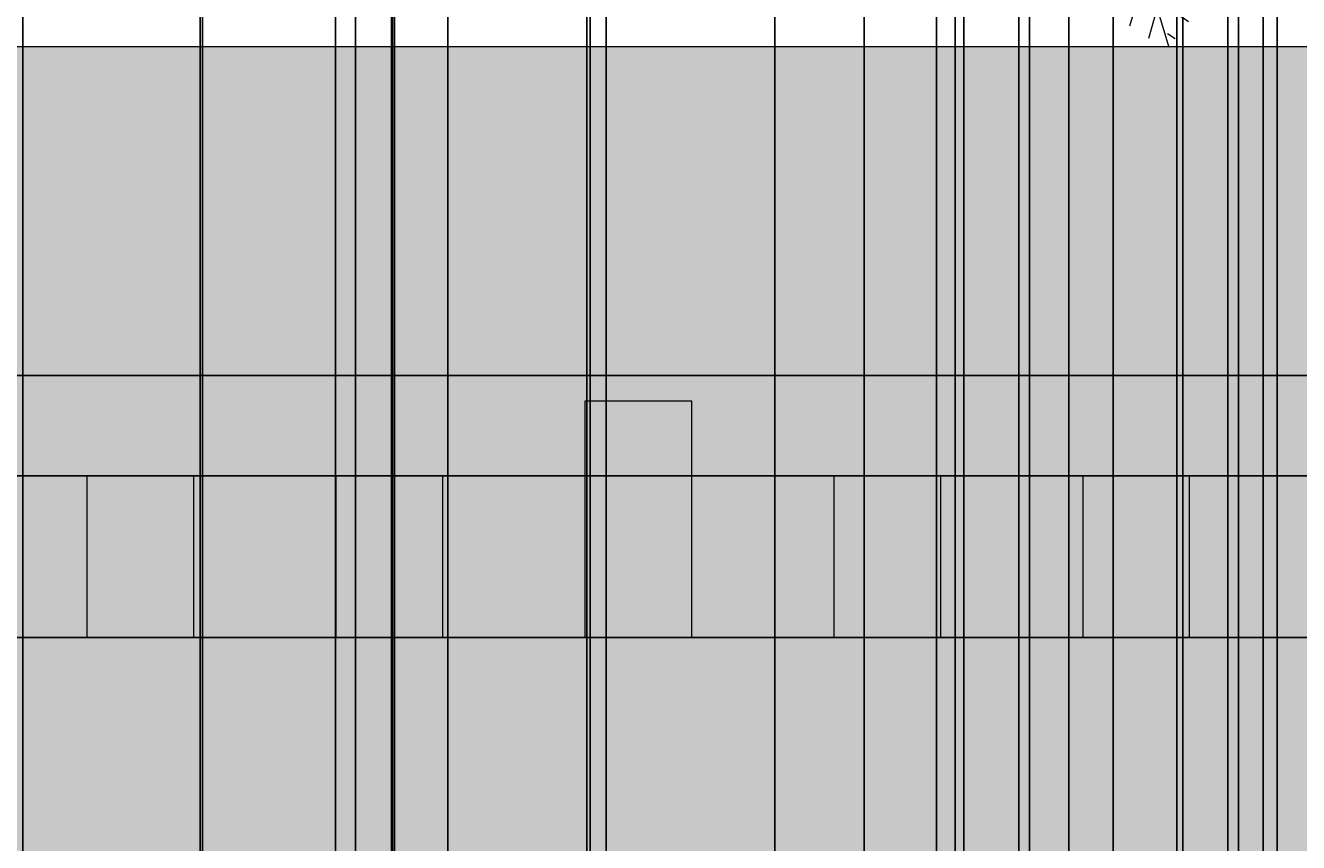
# Model space of a CAD drawing. Units: inches. Extents: x 818 to 1898, y 976 to 2364.
# Tile 80 of 96: x 1259 to 1439, y 2093 to 2209. Entities that reach past the tile are written whole.
import ezdxf

# ---------------------------------------------------------------- set-up
doc = ezdxf.new("R2010")
doc.units = ezdxf.units.IN
doc.header["$LTSCALE"] = 5
doc.header["$MEASUREMENT"] = 0
for name, color, linetype, lineweight in [('A-ANNO-DIMS', 2, 'Continuous', 18), ('L-PAVE', 8, 'Continuous', 18), ('L-PLNT-BEDS', 94, 'Continuous', 18)]:
    doc.layers.add(name, color=color, linetype=linetype, lineweight=lineweight)
for name, color, linetype, lineweight, true_color in [('L-PAVE-PATT', 9, 'Continuous', 9, 0xc7c8ca), ('L-PLNT', 116, 'Continuous', 13, 0x136734), ('L-PLNT-PATT', 114, 'Continuous', 9, 0x139b48)]:
    doc.layers.add(name, color=color, linetype=linetype, lineweight=lineweight, true_color=true_color)
doc.styles.get("Standard").update_dxf_attribs({"font": 'arial.ttf'})
doc.dimstyles.get("Standard").update_dxf_attribs({"dimtxt": 0.18, "dimasz": 0.18, "dimexe": 0.18, "dimexo": 0.0625, "dimgap": 0.09, "dimtad": 0, "dimtih": 1, "dimtoh": 1, "dimdec": 4, "dimzin": 0, "dimdsep": 46, "dimtxsty": 'Standard', "dimcen": 0.09, "dimadec": 0, "dimazin": 0, "dimtfac": 1, "dimtdec": 4, "dimtofl": 0, "dimtmove": 0, "dimatfit": 3, "dimfxl": 1, "dimtolj": 1, "dimtzin": 0, "dimarcsym": 0})

# ---------------------------------------------------------------- blocks, each defined once
blk = doc.blocks.new('PALM-BORDER')
for p, q in [((41.53, 39.05), (33.72, 81.45)), ((33.95, 78.95), (31.8, 80.68)), ((34.76, 77.57), (36.65, 80.68)), ((35.03, 74.11), (28.83, 78.26)), ((35.84, 71.35), (39.61, 75.84)), ((37.18, 65.82), (45, 74.8)), ((36.11, 68.59), (25.33, 73.77)), ((37.72, 59.6), (49.31, 73.77)), ((37.72, 59.95), (23.17, 69.28)), ((39.34, 51.31), (47.96, 67.2)), ((38.8, 53.39), (21.02, 65.48)), ((61.61, 45.75), (77.23, 65.83)), ((61.71, 45.79), (64.67, 65.82)), ((74.37, 66.17), (75.18, 63.4)), ((57.93, 44.41), (61.97, 63.06)), ((67.63, 63.4), (69.25, 55.81)), ((70.33, 64.44), (72.75, 60.3)), ((53.62, 43.37), (58.74, 62.37)), ((65.21, 62.02), (65.75, 51.31)), ((74.1, 61.33), (79.49, 62.02)), ((5.39, 54.77), (4.85, 60.64)), ((9.16, 60.3), (9.97, 50.62)), ((15.09, 59.95), (23.44, 41.99)), ((18.1, 42.4), (2.48, 58.02)), ((12.93, 58.57), (15.63, 44.75)), ((30.72, 40.61), (18.59, 57.88)), ((40.69, 44.06), (48.23, 58.91)), ((49.04, 41.64), (54.7, 58.57)), ((71.68, 58.22), (77.87, 57.53)), ((23.44, 56.84), (39.34, 49.24)), ((44.46, 40.26), (49.85, 57.19)), ((6.2, 53.73), (0, 52.7)), ((68.44, 53.73), (77.33, 52.35)), ((66.29, 51.31), (77.87, 47.17)), ((11.32, 49.24), (0.54, 47.17)), ((26.14, 49.24), (40.69, 42.68)), ((63.59, 48.21), (77.33, 43.71)), ((41.53, 39.05), (61.61, 45.75)), ((16.71, 43.71), (2.69, 43.02)), ((54.97, 43.37), (67.63, 36.46)), ((59.55, 44.75), (76.26, 40.26)), ((20.48, 41.64), (5.93, 34.73)), ((41.53, 39.05), (18.1, 42.4)), ((49.85, 41.64), (64.4, 34.73)), ((25.6, 41.3), (13.2, 33.01)), ((29.64, 40.61), (19.13, 31.97)), ((36.65, 39.91), (25.6, 33.01)), ((46.35, 40.26), (60.9, 32.66)), ((41.53, 39.05), (24.79, 24.55)), ((41.53, 39.05), (54.92, 22.32)), ((37.99, 36.46), (38.8, 28.17)), ((43.38, 36.81), (40.42, 24.02)), ((42.84, 37.15), (59.55, 31.97)), ((36.65, 34.73), (26.68, 31.62)), ((45.27, 34.39), (43.11, 19.88)), ((34.49, 32.66), (36.92, 21.61)), ((47.15, 32.32), (65.48, 28.17)), ((30.18, 29.55), (19.13, 29.55)), ((31.53, 30.59), (35.03, 14.7)), ((48.23, 30.59), (44.19, 12.28)), ((28.56, 27.82), (9.7, 25.06)), ((28.83, 27.82), (32.07, 9.17)), ((50.66, 27.82), (68.98, 25.06)), ((26.14, 25.41), (28.29, 6.06)), ((52, 26.44), (46.35, 9.17)), ((24.79, 24.55), (13.63, 5.58)), ((53.62, 24.37), (68.44, 21.95)), ((23.44, 22.99), (9.97, 22.64)), ((54.97, 22.3), (47.69, 5.02)), ((54.92, 22.32), (61.61, 0)), ((55.24, 22.3), (71.68, 17.46)), ((21.56, 19.53), (11.59, 19.88)), ((22.9, 21.26), (24.52, 5.37)), ((55.78, 20.22), (70.33, 14.35)), ((20.48, 17.46), (9.7, 15.73)), ((56.59, 16.42), (53.35, 5.72)), ((19.94, 16.08), (20.75, 6.41)), ((57.39, 14.7), (70.6, 8.83)), ((18.59, 13.66), (9.97, 12.62)), ((17.24, 11.59), (17.78, 6.06)), ((58.47, 10.9), (56.05, 2.95)), ((15.9, 9.52), (11.05, 7.44)), ((58.47, 10.55), (67.09, 5.72)), ((59.82, 6.75), (64.4, 3.64)), ((59.82, 5.02), (58.74, 1.22)), ((61.44, 1.92), (62.51, 1.22))]:
    blk.add_line(p, q)
blk = doc.blocks.new('*D61')
at = {"layer": 'A-ANNO-DIMS', "color": 0, "lineweight": -2, "ltscale": 5, "transparency": 16777216}
for p, q in [((1071.73, 1203.03), (1071.73, 2363.87)), ((1071.91, 2363.69), (1250.94, 2363.69)), ((1430.55, 2363.69), (1251.51, 2363.69)), ((1430.73, 1203.03), (1430.73, 2363.87))]:
    blk.add_line(p, q, dxfattribs=at)
at = {"layer": 'A-ANNO-DIMS', "color": 0, "ltscale": 5, "transparency": 16777216}
for points in [[(1071.91, 2363.72), (1071.91, 2363.66), (1071.73, 2363.69)], [(1430.55, 2363.72), (1430.55, 2363.66), (1430.73, 2363.69)]]:
    blk.add_solid(points, dxfattribs=at)
at = {"layer": 'Defpoints', "color": 0, "ltscale": 5, "transparency": 16777216}
for p in [(1430.73, 2363.69), (1071.73, 1202.96), (1430.73, 1202.96)]:
    blk.add_point(p, dxfattribs=at)
at = {"layer": 'A-ANNO-DIMS', "color": 0, "ltscale": 5, "transparency": 16777216, "insert": (1251.23, 2363.69), "char_height": 0.18, "attachment_point": 5}
blk.add_mtext('\\A1;359', dxfattribs=at)
blk = doc.blocks.new('*D64')
at = {"layer": 'A-ANNO-DIMS', "color": 0, "lineweight": -2, "ltscale": 5, "transparency": 16777216}
for p, q in [((1197.73, 1501.14), (1197.73, 2363.87)), ((1197.91, 2363.69), (1313.93, 2363.69)), ((1430.55, 2363.69), (1314.52, 2363.69)), ((1430.73, 1501.14), (1430.73, 2363.87))]:
    blk.add_line(p, q, dxfattribs=at)
at = {"layer": 'A-ANNO-DIMS', "color": 0, "ltscale": 5, "transparency": 16777216}
for points in [[(1197.91, 2363.72), (1197.91, 2363.66), (1197.73, 2363.69)], [(1430.55, 2363.72), (1430.55, 2363.66), (1430.73, 2363.69)]]:
    blk.add_solid(points, dxfattribs=at)
at = {"layer": 'Defpoints', "color": 0, "ltscale": 5, "transparency": 16777216}
for p in [(1430.73, 2363.69), (1197.73, 1501.08), (1430.73, 1501.08)]:
    blk.add_point(p, dxfattribs=at)
at = {"layer": 'A-ANNO-DIMS', "color": 0, "ltscale": 5, "transparency": 16777216, "insert": (1314.23, 2363.69), "char_height": 0.18, "attachment_point": 5}
blk.add_mtext('\\A1;233', dxfattribs=at)
blk = doc.blocks.new('*D86')
at = {"layer": 'A-ANNO-DIMS', "color": 0, "lineweight": -2, "ltscale": 5, "transparency": 16777216}
for p, q in [((1258.73, 2053.14), (1258.73, 2363.87)), ((1258.91, 2363.69), (1486.43, 2363.69)), ((1714.55, 2363.69), (1487.02, 2363.69)), ((1714.73, 2053.14), (1714.73, 2363.87))]:
    blk.add_line(p, q, dxfattribs=at)
at = {"layer": 'A-ANNO-DIMS', "color": 0, "ltscale": 5, "transparency": 16777216}
for points in [[(1258.91, 2363.72), (1258.91, 2363.66), (1258.73, 2363.69)], [(1714.55, 2363.72), (1714.55, 2363.66), (1714.73, 2363.69)]]:
    blk.add_solid(points, dxfattribs=at)
at = {"layer": 'Defpoints', "color": 0, "ltscale": 5, "transparency": 16777216}
for p in [(1714.73, 2363.69), (1258.73, 2053.08), (1714.73, 2053.08)]:
    blk.add_point(p, dxfattribs=at)
at = {"layer": 'A-ANNO-DIMS', "color": 0, "ltscale": 5, "transparency": 16777216, "insert": (1486.73, 2363.69), "char_height": 0.18, "attachment_point": 5}
blk.add_mtext('\\A1;456', dxfattribs=at)
blk = doc.blocks.new('*D96')
at = {"layer": 'A-ANNO-DIMS', "color": 0, "lineweight": -2, "ltscale": 5, "transparency": 16777216}
for p, q in [((1229.65, 1071.12), (1229.65, 2363.87)), ((1229.83, 2363.69), (1256.52, 2363.69)), ((1283.99, 2363.69), (1257.3, 2363.69)), ((1284.17, 1071.12), (1284.17, 2363.87))]:
    blk.add_line(p, q, dxfattribs=at)
at = {"layer": 'A-ANNO-DIMS', "color": 0, "ltscale": 5, "transparency": 16777216}
for points in [[(1229.83, 2363.72), (1229.83, 2363.66), (1229.65, 2363.69)], [(1283.99, 2363.72), (1283.99, 2363.66), (1284.17, 2363.69)]]:
    blk.add_solid(points, dxfattribs=at)
at = {"layer": 'Defpoints', "color": 0, "ltscale": 5, "transparency": 16777216}
for p in [(1284.17, 2363.69), (1229.65, 1071.06), (1284.17, 1071.06)]:
    blk.add_point(p, dxfattribs=at)
at = {"layer": 'A-ANNO-DIMS', "color": 0, "ltscale": 5, "transparency": 16777216, "insert": (1256.91, 2363.69), "char_height": 0.18, "attachment_point": 5}
blk.add_mtext('\\A1;54.52', dxfattribs=at)
blk = doc.blocks.new('*D97')
at = {"layer": 'A-ANNO-DIMS', "color": 0, "lineweight": -2, "ltscale": 5, "transparency": 16777216}
for p, q in [((1284.17, 1071.12), (1284.17, 2363.87)), ((1284.35, 2363.69), (1310.96, 2363.69)), ((1338.36, 2363.69), (1311.75, 2363.69)), ((1338.54, 1071.12), (1338.54, 2363.87))]:
    blk.add_line(p, q, dxfattribs=at)
at = {"layer": 'A-ANNO-DIMS', "color": 0, "ltscale": 5, "transparency": 16777216}
for points in [[(1284.35, 2363.72), (1284.35, 2363.66), (1284.17, 2363.69)], [(1338.36, 2363.72), (1338.36, 2363.66), (1338.54, 2363.69)]]:
    blk.add_solid(points, dxfattribs=at)
at = {"layer": 'Defpoints', "color": 0, "ltscale": 5, "transparency": 16777216}
for p in [(1338.54, 2363.69), (1284.17, 1071.06), (1338.54, 1071.06)]:
    blk.add_point(p, dxfattribs=at)
at = {"layer": 'A-ANNO-DIMS', "color": 0, "ltscale": 5, "transparency": 16777216, "insert": (1311.36, 2363.69), "char_height": 0.18, "attachment_point": 5}
blk.add_mtext('\\A1;54.37', dxfattribs=at)
blk = doc.blocks.new('*D98')
at = {"layer": 'A-ANNO-DIMS', "color": 0, "lineweight": -2, "ltscale": 5, "transparency": 16777216}
for p, q in [((1338.54, 1071.12), (1338.54, 2363.87)), ((1338.72, 2363.69), (1364.81, 2363.69)), ((1391.7, 2363.69), (1365.6, 2363.69)), ((1391.88, 1071.12), (1391.88, 2363.87))]:
    blk.add_line(p, q, dxfattribs=at)
at = {"layer": 'A-ANNO-DIMS', "color": 0, "ltscale": 5, "transparency": 16777216}
for points in [[(1338.72, 2363.72), (1338.72, 2363.66), (1338.54, 2363.69)], [(1391.7, 2363.72), (1391.7, 2363.66), (1391.88, 2363.69)]]:
    blk.add_solid(points, dxfattribs=at)
at = {"layer": 'Defpoints', "color": 0, "ltscale": 5, "transparency": 16777216}
for p in [(1391.88, 2363.69), (1338.54, 1071.06), (1391.88, 1071.06)]:
    blk.add_point(p, dxfattribs=at)
at = {"layer": 'A-ANNO-DIMS', "color": 0, "ltscale": 5, "transparency": 16777216, "insert": (1365.21, 2363.69), "char_height": 0.18, "attachment_point": 5}
blk.add_mtext('\\A1;53.33', dxfattribs=at)
blk = doc.blocks.new('*D99')
at = {"layer": 'A-ANNO-DIMS', "color": 0, "lineweight": -2, "ltscale": 5, "transparency": 16777216}
for p, q in [((1391.88, 1071.12), (1391.88, 2363.87)), ((1392.06, 2363.69), (1420.45, 2363.69)), ((1449.64, 2363.69), (1421.24, 2363.69)), ((1449.82, 1071.12), (1449.82, 2363.87))]:
    blk.add_line(p, q, dxfattribs=at)
at = {"layer": 'A-ANNO-DIMS', "color": 0, "ltscale": 5, "transparency": 16777216}
for points in [[(1392.06, 2363.72), (1392.06, 2363.66), (1391.88, 2363.69)], [(1449.64, 2363.72), (1449.64, 2363.66), (1449.82, 2363.69)]]:
    blk.add_solid(points, dxfattribs=at)
at = {"layer": 'Defpoints', "color": 0, "ltscale": 5, "transparency": 16777216}
for p in [(1449.82, 2363.69), (1391.88, 1071.06), (1449.82, 1071.06)]:
    blk.add_point(p, dxfattribs=at)
at = {"layer": 'A-ANNO-DIMS', "color": 0, "ltscale": 5, "transparency": 16777216, "insert": (1420.85, 2363.69), "char_height": 0.18, "attachment_point": 5}
blk.add_mtext('\\A1;57.94', dxfattribs=at)
blk = doc.blocks.new('*D147')
at = {"layer": 'A-ANNO-DIMS', "color": 0, "lineweight": -2, "ltscale": 5, "transparency": 16777216}
for p, q in [((1212.58, 2145.25), (1897.92, 2145.25)), ((1897.74, 2145.07), (1897.74, 2133.99)), ((1897.74, 2122.56), (1897.74, 2133.63)), ((1212.58, 2122.38), (1897.92, 2122.38))]:
    blk.add_line(p, q, dxfattribs=at)
at = {"layer": 'A-ANNO-DIMS', "color": 0, "ltscale": 5, "transparency": 16777216}
for points in [[(1897.71, 2145.07), (1897.77, 2145.07), (1897.74, 2145.25)], [(1897.71, 2122.56), (1897.77, 2122.56), (1897.74, 2122.38)]]:
    blk.add_solid(points, dxfattribs=at)
at = {"layer": 'Defpoints', "color": 0, "ltscale": 5, "transparency": 16777216}
for p in [(1212.52, 2145.25), (1897.74, 2145.25), (1212.52, 2122.38)]:
    blk.add_point(p, dxfattribs=at)
at = {"layer": 'A-ANNO-DIMS', "color": 0, "ltscale": 5, "transparency": 16777216, "insert": (1897.74, 2133.81), "char_height": 0.18, "attachment_point": 5}
blk.add_mtext('\\A1;22.87', dxfattribs=at)
blk = doc.blocks.new('*D148')
at = {"layer": 'A-ANNO-DIMS', "color": 0, "lineweight": -2, "ltscale": 5, "transparency": 16777216}
for p, q in [((1232.67, 2159.43), (1897.92, 2159.43)), ((1897.74, 2159.25), (1897.74, 2141.09)), ((1897.74, 2122.56), (1897.74, 2140.72)), ((1232.67, 2122.38), (1897.92, 2122.38))]:
    blk.add_line(p, q, dxfattribs=at)
at = {"layer": 'A-ANNO-DIMS', "color": 0, "ltscale": 5, "transparency": 16777216}
for points in [[(1897.71, 2159.25), (1897.77, 2159.25), (1897.74, 2159.43)], [(1897.71, 2122.56), (1897.77, 2122.56), (1897.74, 2122.38)]]:
    blk.add_solid(points, dxfattribs=at)
at = {"layer": 'Defpoints', "color": 0, "ltscale": 5, "transparency": 16777216}
for p in [(1232.61, 2159.43), (1897.74, 2159.43), (1232.61, 2122.38)]:
    blk.add_point(p, dxfattribs=at)
at = {"layer": 'A-ANNO-DIMS', "color": 0, "ltscale": 5, "transparency": 16777216, "insert": (1897.74, 2140.9), "char_height": 0.18, "attachment_point": 5}
blk.add_mtext('\\A1;37.05', dxfattribs=at)
blk = doc.blocks.new('*D161')
at = {"layer": 'A-ANNO-DIMS', "color": 0, "lineweight": -2, "ltscale": 5, "transparency": 16777216}
for p, q in [((1429.23, 1876.14), (1429.23, 2363.87)), ((1429.41, 2363.69), (1509.59, 2363.69)), ((1590.55, 2363.69), (1510.36, 2363.69)), ((1590.73, 1876.14), (1590.73, 2363.87))]:
    blk.add_line(p, q, dxfattribs=at)
at = {"layer": 'A-ANNO-DIMS', "color": 0, "ltscale": 5, "transparency": 16777216}
for points in [[(1429.41, 2363.72), (1429.41, 2363.66), (1429.23, 2363.69)], [(1590.55, 2363.72), (1590.55, 2363.66), (1590.73, 2363.69)]]:
    blk.add_solid(points, dxfattribs=at)
at = {"layer": 'Defpoints', "color": 0, "ltscale": 5, "transparency": 16777216}
for p in [(1590.73, 2363.69), (1429.23, 1876.08), (1590.73, 1876.08)]:
    blk.add_point(p, dxfattribs=at)
at = {"layer": 'A-ANNO-DIMS', "color": 0, "ltscale": 5, "transparency": 16777216, "insert": (1509.98, 2363.69), "char_height": 0.18, "attachment_point": 5}
blk.add_mtext('\\A1;161.5', dxfattribs=at)
blk = doc.blocks.new('*D165')
at = {"layer": 'A-ANNO-DIMS', "color": 0, "lineweight": -2, "ltscale": 5, "transparency": 16777216}
for p, q in [((1283.82, 1510.14), (1283.82, 2363.87)), ((1284, 2363.69), (1324.09, 2363.69)), ((1364.97, 2363.69), (1324.88, 2363.69)), ((1365.15, 1510.14), (1365.15, 2363.87))]:
    blk.add_line(p, q, dxfattribs=at)
at = {"layer": 'A-ANNO-DIMS', "color": 0, "ltscale": 5, "transparency": 16777216}
for points in [[(1284, 2363.72), (1284, 2363.66), (1283.82, 2363.69)], [(1364.97, 2363.72), (1364.97, 2363.66), (1365.15, 2363.69)]]:
    blk.add_solid(points, dxfattribs=at)
at = {"layer": 'Defpoints', "color": 0, "ltscale": 5, "transparency": 16777216}
for p in [(1365.15, 2363.69), (1283.82, 1510.08), (1365.15, 1510.08)]:
    blk.add_point(p, dxfattribs=at)
at = {"layer": 'A-ANNO-DIMS', "color": 0, "ltscale": 5, "transparency": 16777216, "insert": (1324.48, 2363.69), "char_height": 0.18, "attachment_point": 5}
blk.add_mtext('\\A1;81.33', dxfattribs=at)
blk = doc.blocks.new('*D166')
at = {"layer": 'A-ANNO-DIMS', "color": 0, "lineweight": -2, "ltscale": 5, "transparency": 16777216}
for p, q in [((1401.15, 1510.14), (1401.15, 2363.87)), ((1401.33, 2363.69), (1415.54, 2363.69)), ((1430.55, 2363.69), (1416.33, 2363.69)), ((1430.73, 1510.14), (1430.73, 2363.87))]:
    blk.add_line(p, q, dxfattribs=at)
at = {"layer": 'A-ANNO-DIMS', "color": 0, "ltscale": 5, "transparency": 16777216}
for points in [[(1401.33, 2363.72), (1401.33, 2363.66), (1401.15, 2363.69)], [(1430.55, 2363.72), (1430.55, 2363.66), (1430.73, 2363.69)]]:
    blk.add_solid(points, dxfattribs=at)
at = {"layer": 'Defpoints', "color": 0, "ltscale": 5, "transparency": 16777216}
for p in [(1430.73, 2363.69), (1401.15, 1510.08), (1430.73, 1510.08)]:
    blk.add_point(p, dxfattribs=at)
at = {"layer": 'A-ANNO-DIMS', "color": 0, "ltscale": 5, "transparency": 16777216, "insert": (1415.94, 2363.69), "char_height": 0.18, "attachment_point": 5}
blk.add_mtext('\\A1;29.58', dxfattribs=at)
blk = doc.blocks.new('*D191')
at = {"layer": 'A-ANNO-DIMS', "color": 0, "lineweight": -2, "ltscale": 5, "transparency": 16777216}
for p, q in [((1434.23, 1409.11), (1434.23, 2363.87)), ((1434.41, 2363.69), (1435.08, 2363.69)), ((1436.05, 2363.69), (1435.37, 2363.69)), ((1436.23, 1409.11), (1436.23, 2363.87))]:
    blk.add_line(p, q, dxfattribs=at)
at = {"layer": 'A-ANNO-DIMS', "color": 0, "ltscale": 5, "transparency": 16777216}
for points in [[(1434.41, 2363.72), (1434.41, 2363.66), (1434.23, 2363.69)], [(1436.05, 2363.72), (1436.05, 2363.66), (1436.23, 2363.69)]]:
    blk.add_solid(points, dxfattribs=at)
at = {"layer": 'Defpoints', "color": 0, "ltscale": 5, "transparency": 16777216}
for p in [(1436.23, 2363.69), (1434.23, 1409.05), (1436.23, 1409.05)]:
    blk.add_point(p, dxfattribs=at)
at = {"layer": 'A-ANNO-DIMS', "color": 0, "ltscale": 5, "transparency": 16777216, "insert": (1435.23, 2363.69), "char_height": 0.18, "attachment_point": 5}
blk.add_mtext('\\A1;2', dxfattribs=at)
blk = doc.blocks.new('*D235')
at = {"layer": 'A-ANNO-DIMS', "color": 0, "lineweight": -2, "ltscale": 5, "transparency": 16777216}
for p, q in [((1310.91, 2026.27), (1310.91, 2363.87)), ((1311.09, 2363.69), (1324.48, 2363.69)), ((1338.81, 2363.69), (1325.41, 2363.69)), ((1338.99, 2026.27), (1338.99, 2363.87))]:
    blk.add_line(p, q, dxfattribs=at)
at = {"layer": 'A-ANNO-DIMS', "color": 0, "ltscale": 5, "transparency": 16777216}
for points in [[(1311.09, 2363.72), (1311.09, 2363.66), (1310.91, 2363.69)], [(1338.81, 2363.72), (1338.81, 2363.66), (1338.99, 2363.69)]]:
    blk.add_solid(points, dxfattribs=at)
at = {"layer": 'Defpoints', "color": 0, "ltscale": 5, "transparency": 16777216}
for p in [(1338.99, 2363.69), (1310.91, 2026.21), (1338.99, 2026.21)]:
    blk.add_point(p, dxfattribs=at)
at = {"layer": 'A-ANNO-DIMS', "color": 0, "ltscale": 5, "transparency": 16777216, "insert": (1324.95, 2363.69), "char_height": 0.18, "attachment_point": 5}
blk.add_mtext('\\A1;28.084', dxfattribs=at)
blk = doc.blocks.new('*D255')
at = {"layer": 'A-ANNO-DIMS', "color": 0, "lineweight": -2, "ltscale": 5, "transparency": 16777216}
for p, q in [((1388.03, 2053.14), (1388.03, 2363.87)), ((1388.21, 2363.69), (1388.94, 2363.69)), ((1390.46, 2363.69), (1389.73, 2363.69)), ((1390.64, 2053.14), (1390.64, 2363.87))]:
    blk.add_line(p, q, dxfattribs=at)
at = {"layer": 'A-ANNO-DIMS', "color": 0, "ltscale": 5, "transparency": 16777216}
for points in [[(1388.21, 2363.72), (1388.21, 2363.66), (1388.03, 2363.69)], [(1390.46, 2363.72), (1390.46, 2363.66), (1390.64, 2363.69)]]:
    blk.add_solid(points, dxfattribs=at)
at = {"layer": 'Defpoints', "color": 0, "ltscale": 5, "transparency": 16777216}
for p in [(1390.64, 2363.69), (1388.03, 2053.08), (1390.64, 2053.08)]:
    blk.add_point(p, dxfattribs=at)
at = {"layer": 'A-ANNO-DIMS', "color": 0, "ltscale": 5, "transparency": 16777216, "insert": (1389.33, 2363.69), "char_height": 0.18, "attachment_point": 5}
blk.add_mtext('\\A1;2.604', dxfattribs=at)
blk = doc.blocks.new('*D256')
at = {"layer": 'A-ANNO-DIMS', "color": 0, "lineweight": -2, "ltscale": 5, "transparency": 16777216}
for p, q in [((1399.64, 2053.14), (1399.64, 2363.87)), ((1399.82, 2363.69), (1405.87, 2363.69)), ((1412.84, 2363.69), (1406.78, 2363.69)), ((1413.02, 2077.25), (1413.02, 2363.87))]:
    blk.add_line(p, q, dxfattribs=at)
at = {"layer": 'A-ANNO-DIMS', "color": 0, "ltscale": 5, "transparency": 16777216}
for points in [[(1399.82, 2363.72), (1399.82, 2363.66), (1399.64, 2363.69)], [(1412.84, 2363.72), (1412.84, 2363.66), (1413.02, 2363.69)]]:
    blk.add_solid(points, dxfattribs=at)
at = {"layer": 'Defpoints', "color": 0, "ltscale": 5, "transparency": 16777216}
for p in [(1413.02, 2363.69), (1413.02, 2077.19), (1399.64, 2053.08)]:
    blk.add_point(p, dxfattribs=at)
at = {"layer": 'A-ANNO-DIMS', "color": 0, "ltscale": 5, "transparency": 16777216, "insert": (1406.33, 2363.69), "char_height": 0.18, "attachment_point": 5}
blk.add_mtext('\\A1;13.384', dxfattribs=at)
blk = doc.blocks.new('*D258')
at = {"layer": 'A-ANNO-DIMS', "color": 0, "lineweight": -2, "ltscale": 5, "transparency": 16777216}
for p, q in [((1422.02, 2053.14), (1422.02, 2363.87)), ((1422.2, 2363.69), (1453.26, 2363.69)), ((1484.94, 2363.69), (1453.88, 2363.69)), ((1485.12, 2053.14), (1485.12, 2363.87))]:
    blk.add_line(p, q, dxfattribs=at)
at = {"layer": 'A-ANNO-DIMS', "color": 0, "ltscale": 5, "transparency": 16777216}
for points in [[(1422.2, 2363.72), (1422.2, 2363.66), (1422.02, 2363.69)], [(1484.94, 2363.72), (1484.94, 2363.66), (1485.12, 2363.69)]]:
    blk.add_solid(points, dxfattribs=at)
at = {"layer": 'Defpoints', "color": 0, "ltscale": 5, "transparency": 16777216}
for p in [(1485.12, 2363.69), (1422.02, 2053.08), (1485.12, 2053.08)]:
    blk.add_point(p, dxfattribs=at)
at = {"layer": 'A-ANNO-DIMS', "color": 0, "ltscale": 5, "transparency": 16777216, "insert": (1453.57, 2363.69), "char_height": 0.18, "attachment_point": 5}
blk.add_mtext('\\A1;63.1', dxfattribs=at)
blk = doc.blocks.new('*D269')
at = {"layer": 'A-ANNO-DIMS', "color": 0, "lineweight": -2, "ltscale": 5, "transparency": 16777216}
for p, q in [((1246.94, 1534.14), (1246.94, 2363.87)), ((1247.12, 2363.69), (1293.71, 2363.69)), ((1341.08, 2363.69), (1294.49, 2363.69)), ((1341.26, 1534.14), (1341.26, 2363.87))]:
    blk.add_line(p, q, dxfattribs=at)
at = {"layer": 'A-ANNO-DIMS', "color": 0, "ltscale": 5, "transparency": 16777216}
for points in [[(1247.12, 2363.72), (1247.12, 2363.66), (1246.94, 2363.69)], [(1341.08, 2363.72), (1341.08, 2363.66), (1341.26, 2363.69)]]:
    blk.add_solid(points, dxfattribs=at)
at = {"layer": 'Defpoints', "color": 0, "ltscale": 5, "transparency": 16777216}
for p in [(1341.26, 2363.69), (1246.94, 1534.08), (1341.26, 1534.08)]:
    blk.add_point(p, dxfattribs=at)
at = {"layer": 'A-ANNO-DIMS', "color": 0, "ltscale": 5, "transparency": 16777216, "insert": (1294.1, 2363.69), "char_height": 0.18, "attachment_point": 5}
blk.add_mtext('\\A1;94.32', dxfattribs=at)
blk = doc.blocks.new('*D273')
at = {"layer": 'A-ANNO-DIMS', "color": 0, "lineweight": -2, "ltscale": 5, "transparency": 16777216}
for p, q in [((1406.73, 1587.48), (1406.73, 2363.87)), ((1406.91, 2363.69), (1418.51, 2363.69)), ((1430.55, 2363.69), (1418.95, 2363.69)), ((1430.73, 1587.48), (1430.73, 2363.87))]:
    blk.add_line(p, q, dxfattribs=at)
at = {"layer": 'A-ANNO-DIMS', "color": 0, "ltscale": 5, "transparency": 16777216}
for points in [[(1406.91, 2363.72), (1406.91, 2363.66), (1406.73, 2363.69)], [(1430.55, 2363.72), (1430.55, 2363.66), (1430.73, 2363.69)]]:
    blk.add_solid(points, dxfattribs=at)
at = {"layer": 'Defpoints', "color": 0, "ltscale": 5, "transparency": 16777216}
for p in [(1430.73, 2363.69), (1406.73, 1587.42), (1430.73, 1587.42)]:
    blk.add_point(p, dxfattribs=at)
at = {"layer": 'A-ANNO-DIMS', "color": 0, "ltscale": 5, "transparency": 16777216, "insert": (1418.73, 2363.69), "char_height": 0.18, "attachment_point": 5}
blk.add_mtext('\\A1;24', dxfattribs=at)
blk = doc.blocks.new('*D274')
at = {"layer": 'A-ANNO-DIMS', "color": 0, "lineweight": -2, "ltscale": 5, "transparency": 16777216}
for p, q in [((1311.03, 1897.93), (1311.03, 2363.87)), ((1311.21, 2363.69), (1344.01, 2363.69)), ((1377.6, 2363.69), (1344.8, 2363.69)), ((1377.78, 1897.93), (1377.78, 2363.87))]:
    blk.add_line(p, q, dxfattribs=at)
at = {"layer": 'A-ANNO-DIMS', "color": 0, "ltscale": 5, "transparency": 16777216}
for points in [[(1311.21, 2363.72), (1311.21, 2363.66), (1311.03, 2363.69)], [(1377.6, 2363.72), (1377.6, 2363.66), (1377.78, 2363.69)]]:
    blk.add_solid(points, dxfattribs=at)
at = {"layer": 'Defpoints', "color": 0, "ltscale": 5, "transparency": 16777216}
for p in [(1377.78, 2363.69), (1311.03, 1897.87), (1377.78, 1897.87)]:
    blk.add_point(p, dxfattribs=at)
at = {"layer": 'A-ANNO-DIMS', "color": 0, "ltscale": 5, "transparency": 16777216, "insert": (1344.4, 2363.69), "char_height": 0.18, "attachment_point": 5}
blk.add_mtext('\\A1;66.75', dxfattribs=at)
blk = doc.blocks.new('*D281')
at = {"layer": 'A-ANNO-DIMS', "color": 0, "lineweight": -2, "ltscale": 5, "transparency": 16777216}
for p, q in [((1250.3, 1913.7), (1250.3, 2363.87)), ((1250.48, 2363.69), (1420.12, 2363.69)), ((1590.55, 2363.69), (1420.91, 2363.69)), ((1590.73, 2011.14), (1590.73, 2363.87))]:
    blk.add_line(p, q, dxfattribs=at)
at = {"layer": 'A-ANNO-DIMS', "color": 0, "ltscale": 5, "transparency": 16777216}
for points in [[(1250.48, 2363.72), (1250.48, 2363.66), (1250.3, 2363.69)], [(1590.55, 2363.72), (1590.55, 2363.66), (1590.73, 2363.69)]]:
    blk.add_solid(points, dxfattribs=at)
at = {"layer": 'Defpoints', "color": 0, "ltscale": 5, "transparency": 16777216}
for p in [(1590.73, 2363.69), (1590.73, 2011.08), (1250.3, 1913.64)]:
    blk.add_point(p, dxfattribs=at)
at = {"layer": 'A-ANNO-DIMS', "color": 0, "ltscale": 5, "transparency": 16777216, "insert": (1420.51, 2363.69), "char_height": 0.18, "attachment_point": 5}
blk.add_mtext('\\A1;340.4', dxfattribs=at)
blk = doc.blocks.new('*D286')
at = {"layer": 'A-ANNO-DIMS', "color": 0, "lineweight": -2, "ltscale": 5, "transparency": 16777216}
for p, q in [((1305.83, 1851.97), (1305.83, 2363.87)), ((1306.01, 2363.69), (1308.18, 2363.69)), ((1311.15, 2363.69), (1308.97, 2363.69)), ((1311.33, 1853.81), (1311.33, 2363.87))]:
    blk.add_line(p, q, dxfattribs=at)
at = {"layer": 'A-ANNO-DIMS', "color": 0, "ltscale": 5, "transparency": 16777216}
for points in [[(1306.01, 2363.72), (1306.01, 2363.66), (1305.83, 2363.69)], [(1311.15, 2363.72), (1311.15, 2363.66), (1311.33, 2363.69)]]:
    blk.add_solid(points, dxfattribs=at)
at = {"layer": 'Defpoints', "color": 0, "ltscale": 5, "transparency": 16777216}
for p in [(1305.83, 2363.69), (1311.33, 1853.75), (1305.83, 1851.91)]:
    blk.add_point(p, dxfattribs=at)
at = {"layer": 'A-ANNO-DIMS', "color": 0, "ltscale": 5, "transparency": 16777216, "insert": (1308.58, 2363.69), "char_height": 0.18, "attachment_point": 5}
blk.add_mtext('\\A1;5.499', dxfattribs=at)
blk = doc.blocks.new('*D288')
at = {"layer": 'A-ANNO-DIMS', "color": 0, "lineweight": -2, "ltscale": 5, "transparency": 16777216}
for p, q in [((1422.88, 1742.67), (1422.88, 2363.87)), ((1423.06, 2363.69), (1466.91, 2363.69)), ((1511.55, 2363.69), (1467.69, 2363.69)), ((1511.73, 1716.11), (1511.73, 2363.87))]:
    blk.add_line(p, q, dxfattribs=at)
at = {"layer": 'A-ANNO-DIMS', "color": 0, "ltscale": 5, "transparency": 16777216}
for points in [[(1423.06, 2363.72), (1423.06, 2363.66), (1422.88, 2363.69)], [(1511.55, 2363.72), (1511.55, 2363.66), (1511.73, 2363.69)]]:
    blk.add_solid(points, dxfattribs=at)
at = {"layer": 'Defpoints', "color": 0, "ltscale": 5, "transparency": 16777216}
for p in [(1511.73, 2363.69), (1422.88, 1742.61), (1511.73, 1716.05)]:
    blk.add_point(p, dxfattribs=at)
at = {"layer": 'A-ANNO-DIMS', "color": 0, "ltscale": 5, "transparency": 16777216, "insert": (1467.3, 2363.69), "char_height": 0.18, "attachment_point": 5}
blk.add_mtext('\\A1;88.85', dxfattribs=at)
blk = doc.blocks.new('*D290')
at = {"layer": 'A-ANNO-DIMS', "color": 0, "lineweight": -2, "ltscale": 5, "transparency": 16777216}
for p, q in [((1302.98, 1599.43), (1302.98, 2363.87)), ((1303.16, 2363.69), (1310.57, 2363.69)), ((1318.71, 2363.69), (1311.31, 2363.69)), ((1318.89, 1607.83), (1318.89, 2363.87))]:
    blk.add_line(p, q, dxfattribs=at)
at = {"layer": 'A-ANNO-DIMS', "color": 0, "ltscale": 5, "transparency": 16777216}
for points in [[(1303.16, 2363.72), (1303.16, 2363.66), (1302.98, 2363.69)], [(1318.71, 2363.72), (1318.71, 2363.66), (1318.89, 2363.69)]]:
    blk.add_solid(points, dxfattribs=at)
at = {"layer": 'Defpoints', "color": 0, "ltscale": 5, "transparency": 16777216}
for p in [(1318.89, 2363.69), (1318.89, 1607.77), (1302.98, 1599.37)]:
    blk.add_point(p, dxfattribs=at)
at = {"layer": 'A-ANNO-DIMS', "color": 0, "ltscale": 5, "transparency": 16777216, "insert": (1310.94, 2363.69), "char_height": 0.18, "attachment_point": 5}
blk.add_mtext('\\A1;15.91', dxfattribs=at)

msp = doc.modelspace()

# ---------------------------------------------------------------- hatches: boundary and pattern name
at = {"layer": 'L-PAVE-PATT', "ltscale": 5}
h = msp.add_hatch(color=256, dxfattribs=at)
h.dxf.hatch_style = 1
h.paths.add_polyline_path([(1212.5206, 2145.2461), (1197.3925, 2145.2461), (1197.3925, 2122.3767), (1212.5206, 2122.3767)])
h.paths.add_polyline_path([(1247.7373, 2159.4296), (1232.6091, 2159.4296), (1232.6091, 2122.3767), (1247.7373, 2122.3767)])
h.paths.add_polyline_path([(1282.9539, 2145.2461), (1267.8258, 2145.2461), (1267.8258, 2122.3767), (1282.9539, 2122.3767)])
h.paths.add_polyline_path([(1318.1705, 2145.2461), (1303.0424, 2145.2461), (1303.0424, 2122.3767), (1318.1705, 2122.3767)])
h.paths.add_polyline_path([(1353.3871, 2155.7839), (1338.259, 2155.7839), (1338.259, 2122.3767), (1353.3871, 2122.3767)])
h.paths.add_polyline_path([(1388.6037, 2145.2461), (1373.4756, 2145.2461), (1373.4756, 2122.3767), (1388.6037, 2122.3767)])
h.paths.add_polyline_path([(1423.8203, 2145.2461), (1408.6922, 2145.2461), (1408.6922, 2122.3767), (1423.8203, 2122.3767)])
h.paths.add_polyline_path([(1459.037, 2158.4222), (1443.9089, 2158.4222), (1443.9089, 2122.3767), (1459.037, 2122.3767)])
h.paths.add_polyline_path([(1494.2536, 2145.2461), (1479.1255, 2145.2461), (1479.1255, 2122.3767), (1494.2536, 2122.3767)])
h.paths.add_polyline_path([(1529.4702, 2145.2461), (1514.3421, 2145.2461), (1514.3421, 2122.3767), (1529.4702, 2122.3767)])
h.paths.add_polyline_path([(1564.6868, 2156.9246), (1549.5587, 2156.9246), (1549.5587, 2122.3767), (1564.6868, 2122.3767)])
h.paths.add_polyline_path([(1599.9034, 2145.2461), (1584.7753, 2145.2461), (1584.7753, 2122.3767), (1599.9034, 2122.3767)])
h.paths.add_polyline_path([(1635.1201, 2145.2461), (1619.9919, 2145.2461), (1619.9919, 2122.3767), (1635.1201, 2122.3767)])
h.paths.add_polyline_path([(1670.3367, 2156.1761), (1655.2086, 2156.1761), (1655.2086, 2122.3767), (1670.3367, 2122.3767)])
h.paths.add_polyline_path([(1701.7273, 2145.2461), (1686.5992, 2145.2461), (1686.5992, 2122.3767), (1701.7273, 2122.3767)])
h.paths.add_polyline_path([(1730.8897, 2145.2461), (1715.7616, 2145.2461), (1715.7616, 2122.3767), (1730.8897, 2122.3767)])
h.paths.add_polyline_path([(1776.3312, 2145.2461), (1753.1652, 2145.2461), (1753.1652, 2115.6891), (1776.3312, 2115.6891)])
at = {"layer": 'L-PLNT-PATT', "ltscale": 5}
h = msp.add_hatch(color=256, dxfattribs=at)
h.dxf.hatch_style = 1
h.paths.add_polyline_path([(1789.7173, 2205.9709), (1083.7252, 2205.9709), (1083.7252, 2083.2623), (1218.1114, 2083.2623), (1218.1114, 2053.0782), (1390.6356, 2053.0782), (1390.6356, 2081.1881), (1399.6356, 2081.1881), (1413.02, 2081.1881), (1422.02, 2081.1881), (1422.02, 2053.0782), (1676.6446, 2053.0782), (1676.6446, 2081.1881), (1714.7251, 2081.1881), (1714.7251, 2081.6235), (1789.7173, 2081.6235)])
h.paths.add_polyline_path([(1388.6037, 2145.2461), (1388.6037, 2122.3767), (1373.4756, 2122.3767), (1373.4756, 2145.2461)], flags=16)
h.paths.add_polyline_path([(1408.6922, 2145.2461), (1423.8203, 2145.2461), (1423.8203, 2122.3767), (1408.6922, 2122.3767)], flags=16)
h.paths.add_polyline_path([(1353.3871, 2155.7839), (1353.3871, 2122.3767), (1338.259, 2122.3767), (1338.259, 2155.7839)], flags=16)
h.paths.add_polyline_path([(1443.9089, 2158.4222), (1459.037, 2158.4222), (1459.037, 2122.3767), (1443.9089, 2122.3767)], flags=16)
h.paths.add_polyline_path([(1318.1705, 2145.2461), (1318.1705, 2122.3767), (1303.0424, 2122.3767), (1303.0424, 2145.2461)], flags=16)
h.paths.add_polyline_path([(1479.1255, 2145.2461), (1494.2536, 2145.2461), (1494.2536, 2122.3767), (1479.1255, 2122.3767)], flags=16)
h.paths.add_polyline_path([(1282.9539, 2145.2461), (1282.9539, 2122.3767), (1267.8258, 2122.3767), (1267.8258, 2145.2461)], flags=16)
h.paths.add_polyline_path([(1514.3421, 2145.2461), (1529.4702, 2145.2461), (1529.4702, 2122.3767), (1514.3421, 2122.3767)], flags=16)
h.paths.add_polyline_path([(1247.7373, 2159.4296), (1247.7373, 2122.3767), (1232.6091, 2122.3767), (1232.6091, 2159.4296)], flags=16)
h.paths.add_polyline_path([(1549.5587, 2156.9246), (1564.6868, 2156.9246), (1564.6868, 2122.3767), (1549.5587, 2122.3767)], flags=16)
h.paths.add_polyline_path([(1212.5206, 2145.2461), (1212.5206, 2122.3767), (1197.3925, 2122.3767), (1197.3925, 2145.2461)], flags=16)
h.paths.add_polyline_path([(1584.7753, 2145.2461), (1599.9034, 2145.2461), (1599.9034, 2122.3767), (1584.7753, 2122.3767)], flags=16)
h.paths.add_polyline_path([(1185.1073, 2104.7786), (1190.6407, 2104.7786), (1185.1073, 2098.2505), (1179.5738, 2104.7786)], flags=16)
h.paths.add_polyline_path([(1619.9919, 2145.2461), (1635.1201, 2145.2461), (1635.1201, 2122.3767), (1619.9919, 2122.3767)], flags=16)
h.paths.add_polyline_path([(1655.2086, 2156.1761), (1670.3367, 2156.1761), (1670.3367, 2122.3767), (1655.2086, 2122.3767)], flags=16)
h.paths.add_polyline_path([(1686.5992, 2145.2461), (1701.7273, 2145.2461), (1701.7273, 2122.3767), (1686.5992, 2122.3767)], flags=16)
h.paths.add_polyline_path([(1715.7616, 2145.2461), (1730.8897, 2145.2461), (1730.8897, 2122.3767), (1715.7616, 2122.3767)], flags=16)
h.paths.add_polyline_path([(1753.1652, 2145.2461), (1776.3312, 2145.2461), (1776.3312, 2115.6891), (1753.1652, 2115.6891)], flags=16)
h.paths.add_polyline_path([(1191.4331, 2146.5159), (1176.7891, 2146.5159), (1176.7891, 2134.1516), (1191.4331, 2134.1516)], flags=24)

# ---------------------------------------------------------------- linework, layer by layer
at = {"layer": 'L-PAVE', "ltscale": 5}
for points in [[(1353.3871, 2155.7839), (1338.259, 2155.7839), (1338.259, 2122.3767), (1353.3871, 2122.3767)], [(1282.9539, 2145.2461), (1267.8258, 2145.2461), (1267.8258, 2122.3767), (1282.9539, 2122.3767)], [(1318.1705, 2145.2461), (1303.0424, 2145.2461), (1303.0424, 2122.3767), (1318.1705, 2122.3767)], [(1388.6037, 2145.2461), (1373.4756, 2145.2461), (1373.4756, 2122.3767), (1388.6037, 2122.3767)], [(1423.8203, 2145.2461), (1408.6922, 2145.2461), (1408.6922, 2122.3767), (1423.8203, 2122.3767)]]:
    msp.add_lwpolyline(points, close=True, dxfattribs=at)
at = {"layer": 'L-PLNT-BEDS', "ltscale": 5}
msp.add_line((1789.7173, 2205.9709), (1083.7252, 2205.9709), dxfattribs=at)

# ---------------------------------------------------------------- block references
at = {"layer": 'L-PLNT'}
msp.add_blockref('PALM-BORDER', (1359.2483, 2205.9177), dxfattribs=at)

# ---------------------------------------------------------------- dimensions: what is measured, and where the dimension line sits
at = {"layer": 'A-ANNO-DIMS', "ltscale": 5}
for base, p1, p2, override, picture, middle in [((1430.7251, 2363.6929), (1071.7251, 1202.9642), (1430.7251, 1202.9642), {"dimdec": 0, "dimlfac": 1, "dimrnd": 0, "dimzin": 0, "dimdsep": 46, "dimlunit": 2}, '*D61', (1251.2251, 2363.6929)), ((1430.7251, 2363.6929), (1197.7251, 1501.0782), (1430.7251, 1501.0782), {"dimdec": 0, "dimlfac": 1, "dimrnd": 0, "dimzin": 0, "dimdsep": 46, "dimlunit": 2}, '*D64', (1314.2251, 2363.6929)), ((1284.1697, 2363.6929), (1229.6474, 1071.0552), (1284.1697, 1071.0552), {"dimdec": 2, "dimlfac": 1, "dimrnd": 0, "dimzin": 0, "dimdsep": 46, "dimlunit": 2}, '*D96', (1256.9085, 2363.6929)), ((1341.2593, 2363.6929), (1246.9377, 1534.0782), (1341.2593, 1534.0782), {"dimdec": 2, "dimlfac": 1, "dimrnd": 0, "dimzin": 0, "dimdsep": 46, "dimlunit": 2}, '*D269', (1294.0985, 2363.6929)), ((1590.7251, 2363.6929), (1250.3029, 1913.6401), (1590.7251, 2011.0782), {"dimdec": 1, "dimlfac": 1, "dimrnd": 0, "dimzin": 0, "dimdsep": 46, "dimlunit": 2}, '*D281', (1420.514, 2363.6929)), ((1714.7251, 2363.6929), (1258.7251, 2053.0782), (1714.7251, 2053.0782), {"dimdec": 0, "dimlfac": 1, "dimrnd": 0, "dimzin": 0, "dimdsep": 46, "dimlunit": 2}, '*D86', (1486.7251, 2363.6929)), ((1365.1463, 2363.6929), (1283.8183, 1510.0782), (1365.1463, 1510.0782), {"dimdec": 2, "dimlfac": 1, "dimrnd": 0, "dimzin": 0, "dimdsep": 46, "dimlunit": 2}, '*D165', (1324.4823, 2363.6929)), ((1338.5412, 2363.6929), (1284.1697, 1071.0552), (1338.5412, 1071.0552), {"dimdec": 2, "dimlfac": 1, "dimrnd": 0, "dimzin": 0, "dimdsep": 46, "dimlunit": 2}, '*D97', (1311.3554, 2363.6929)), ((1318.8931, 2363.6929), (1302.9835, 1599.3725), (1318.8931, 1607.7707), {"dimdec": 2, "dimlfac": 1, "dimrnd": 0, "dimzin": 0, "dimdsep": 46, "dimlunit": 2}, '*D290', (1310.9383, 2363.6929)), ((1305.8278, 2363.6929), (1311.3271, 1853.7496), (1305.8278, 1851.9081), {"dimdec": 3, "dimlfac": 1, "dimrnd": 0, "dimzin": 0, "dimdsep": 46, "dimlunit": 2}, '*D286', (1308.5774, 2363.6929)), ((1338.9915, 2363.6929), (1310.9077, 2026.2074), (1338.9915, 2026.2074), {"dimdec": 3, "dimlfac": 1, "dimrnd": 0, "dimzin": 0, "dimdsep": 46, "dimlunit": 2}, '*D235', (1324.9496, 2363.6929)), ((1377.7791, 2363.6929), (1311.025, 1897.8663), (1377.7791, 1897.8663), {"dimdec": 2, "dimlfac": 1, "dimrnd": 0, "dimzin": 0, "dimdsep": 46, "dimlunit": 2}, '*D274', (1344.4021, 2363.6929)), ((1391.8757, 2363.6929), (1338.5412, 1071.0552), (1391.8757, 1071.0552), {"dimdec": 2, "dimlfac": 1, "dimrnd": 0, "dimzin": 0, "dimdsep": 46, "dimlunit": 2}, '*D98', (1365.2084, 2363.6929)), ((1390.6356, 2363.6929), (1388.0315, 2053.0782), (1390.6356, 2053.0782), {"dimdec": 3, "dimlfac": 1, "dimrnd": 0, "dimzin": 0, "dimdsep": 46, "dimlunit": 2}, '*D255', (1389.3335, 2363.6929)), ((1449.8196, 2363.6929), (1391.8757, 1071.0552), (1449.8196, 1071.0552), {"dimdec": 2, "dimlfac": 1, "dimrnd": 0, "dimzin": 0, "dimdsep": 46, "dimlunit": 2}, '*D99', (1420.8477, 2363.6929)), ((1413.02, 2363.6929), (1399.6356, 2053.0782), (1413.02, 2077.1881), {"dimdec": 3, "dimlfac": 1, "dimrnd": 0, "dimzin": 0, "dimdsep": 46, "dimlunit": 2}, '*D256', (1406.3278, 2363.6929)), ((1430.7251, 2363.6929), (1401.1463, 1510.0782), (1430.7251, 1510.0782), {"dimdec": 2, "dimlfac": 1, "dimrnd": 0, "dimzin": 0, "dimdsep": 46, "dimlunit": 2}, '*D166', (1415.9357, 2363.6929)), ((1430.7251, 2363.6929), (1406.7251, 1587.4164), (1430.7251, 1587.4164), {"dimdec": 0, "dimlfac": 1, "dimrnd": 0, "dimzin": 0, "dimdsep": 46, "dimlunit": 2}, '*D273', (1418.7251, 2363.6929)), ((1485.1216, 2363.6929), (1422.02, 2053.0782), (1485.1216, 2053.0782), {"dimdec": 1, "dimlfac": 1, "dimrnd": 0, "dimzin": 0, "dimdsep": 46, "dimlunit": 2}, '*D258', (1453.5708, 2363.6929)), ((1511.7251, 2363.6929), (1422.8756, 1742.6113), (1511.7251, 1716.0454), {"dimdec": 2, "dimlfac": 1, "dimrnd": 0, "dimzin": 0, "dimdsep": 46, "dimlunit": 2}, '*D288', (1467.3004, 2363.6929)), ((1590.7251, 2363.6929), (1429.2251, 1876.0782), (1590.7251, 1876.0782), {"dimdec": 1, "dimlfac": 1, "dimrnd": 0, "dimzin": 0, "dimdsep": 46, "dimlunit": 2}, '*D161', (1509.9751, 2363.6929)), ((1436.2251, 2363.6929), (1434.2251, 1409.0522), (1436.2251, 1409.0522), {"dimdec": 0, "dimlfac": 1, "dimrnd": 0, "dimzin": 0, "dimdsep": 46, "dimlunit": 2}, '*D191', (1435.2251, 2363.6929))]:
    dim = msp.add_linear_dim(base=base, p1=p1, p2=p2, dimstyle='Standard', override=override, dxfattribs=at)
    dim.commit()
    dim.dimension.update_dxf_attribs({"geometry": picture, "text_midpoint": middle})
for base, p1, p2, picture, middle in [((1897.736, 2159.4296), (1232.6091, 2122.3767), (1232.6091, 2159.4296), '*D148', (1897.736, 2140.9032)), ((1897.736, 2145.2461), (1212.5206, 2122.3767), (1212.5206, 2145.2461), '*D147', (1897.736, 2133.8114))]:
    dim = msp.add_linear_dim(base=base, p1=p1, p2=p2, angle=90, dimstyle='Standard', override={"dimdec": 2, "dimlfac": 1, "dimrnd": 0, "dimzin": 0, "dimdsep": 46, "dimlunit": 2}, dxfattribs=at)
    dim.commit()
    dim.dimension.update_dxf_attribs({"geometry": picture, "text_midpoint": middle})

doc.saveas('drawing.dxf')
